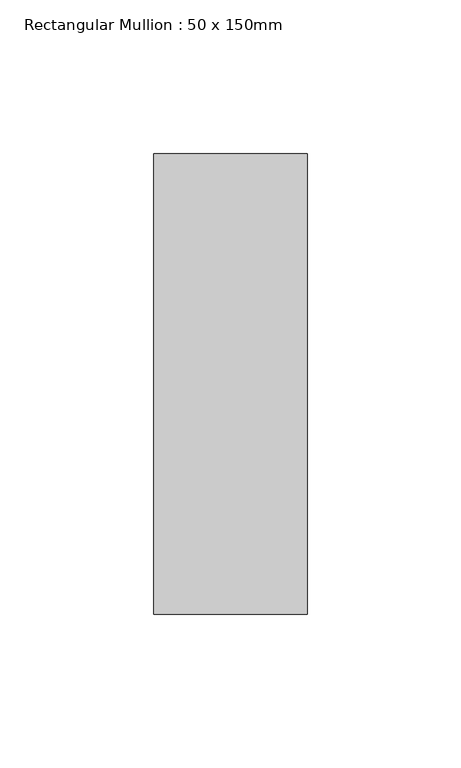
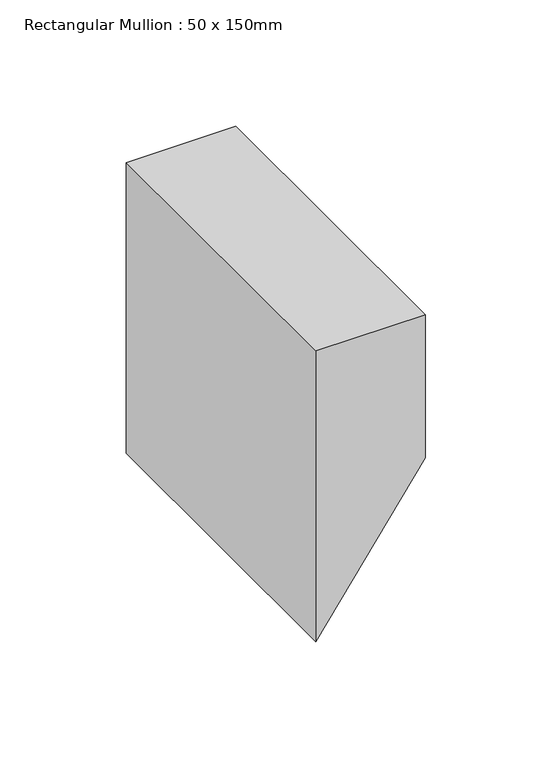
"""IFC4 building model written with IfcOpenShell, lengths in millimetres: member geometry, Rectangular Mullion : 50 x 150mm."""

from ifc_helpers import new_model, si_unit, frame, origin, place, context, project, spatial, polyline, outline, extrude, source, transform, mapped, element, save


def rectangular_mullion_50_x_150mm_e512abdd(model_context):
    return source(origin(), model_context, "Body", "SweptSolid", [
        extrude(outline(polyline([(0.0, 25.0), (0.0, -25.0), (-140.4413185, -25.0), (-69.0339182, 25.0), (0.0, 25.0)])), frame((0.0, -75.0, 0.0), z_axis=(0.0, 1.0, 0.0), x_axis=(0.0, 0.0, 1.0)), (0.0, 0.0, 1.0), 150.0),
    ])


if __name__ == "__main__":
    model = new_model("IFC4")
    model_context = context("Model", 3, world=origin())
    ifc_project = project(units=[si_unit("LENGTHUNIT", "METRE", prefix="MILLI")], contexts=[model_context])
    site = spatial("IfcSite", under=ifc_project)
    building = spatial("IfcBuilding", under=site)
    placement = place(None, origin())
    rectangular_mullion_50_x_150mm_shape = rectangular_mullion_50_x_150mm_e512abdd(model_context)
    element("IfcMember", 1, ObjectType="Rectangular Mullion : 50 x 150mm", at=placement, inside=building, context=model_context, shape_type="MappedRepresentation", body=[
        mapped(rectangular_mullion_50_x_150mm_shape, transform((0.0, 0.0, 0.0), x_axis=(1.0, 0.0, 0.0), y_axis=(0.0, 1.0, 0.0), z_axis=(0.0, 0.0, 1.0))),
    ])
    save(model, "model.ifc")

# Revit data of these elements
# Type "Rectangular Mullion : 50 x 150mm"
#   built-in parameter 1007304 = 0.492126 (stored number, unit not read)
#   built-in parameter 1007301 = 0.082021 (stored number, unit not read)
#   built-in parameter 1007300 = 0.082021 (stored number, unit not read)
# Element 1 (IfcMember, "Rectangular Mullion : 50 x 150mm")
#   Materials on its faces: "Aluminium"
# Materials
#   "Aluminium": class "Metal", colour RGB 247 247 247, transparency 0, Description = "Aluminium 6061", Cost = 0
